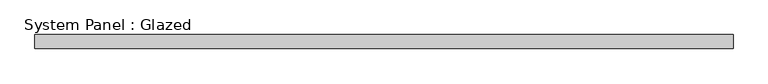
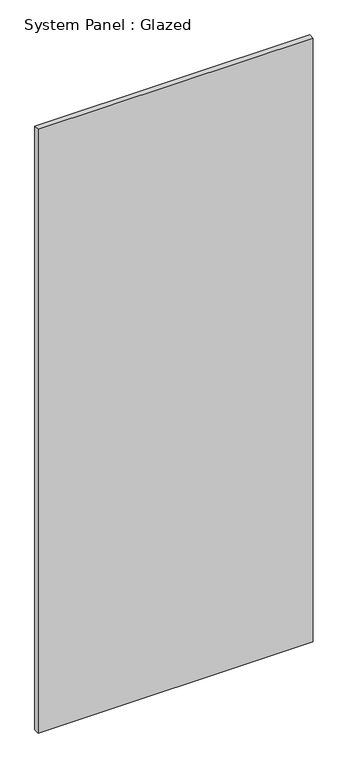
"""IFC4 building model written with IfcOpenShell, lengths in millimetres: plate geometry, System Panel : Glazed."""

from ifc_helpers import new_model, si_unit, origin, origin_with_axes, place, context, project, spatial, polyline, outline, extrude, source, transform, mapped, element, save


def system_panel_glazed_f492b607(model_context):
    return source(origin(), model_context, "Body", "SweptSolid", [
        extrude(outline(polyline([(629.66273, 19.05), (-629.66273, 19.05), (-629.66273, 44.45), (629.66273, 44.45), (629.66273, 19.05)])), origin_with_axes(), (0.0, 0.0, 1.0), 2921.0),
    ])


if __name__ == "__main__":
    model = new_model("IFC4")
    model_context = context("Model", 3, world=origin())
    ifc_project = project(units=[si_unit("LENGTHUNIT", "METRE", prefix="MILLI")], contexts=[model_context])
    site = spatial("IfcSite", under=ifc_project)
    building = spatial("IfcBuilding", under=site)
    placement = place(None, origin())
    system_panel_glazed_shape = system_panel_glazed_f492b607(model_context)
    element("IfcPlate", 1, ObjectType="System Panel : Glazed", at=placement, inside=building, context=model_context, shape_type="MappedRepresentation", body=[
        mapped(system_panel_glazed_shape, transform((0.0, 0.0, 0.0), x_axis=(1.0, 0.0, 0.0), y_axis=(0.0, 1.0, 0.0), z_axis=(0.0, 0.0, 1.0))),
    ])
    save(model, "model.ifc")

# Revit data of these elements
# Type "System Panel : Glazed"
#   Construction Type Id = "GSP4R"
#   Analytic Construction = "1/8 in Pilkington single glazing"
#   Visual Light Transmittance = 0.9
#   Solar Heat Gain Coefficient = 0.86
#   Heat Transfer Coefficient (U) = 1.18115 BTU/(h·ft²·°F)
# Element 1 (IfcPlate, "System Panel : Glazed")
#   Materials on its faces: "Glass"
# Materials
#   "Glass": class "Glass", colour RGB 0 128 192, transparency 0.75, Description = "Soda Lime Glass", Cost = 0
